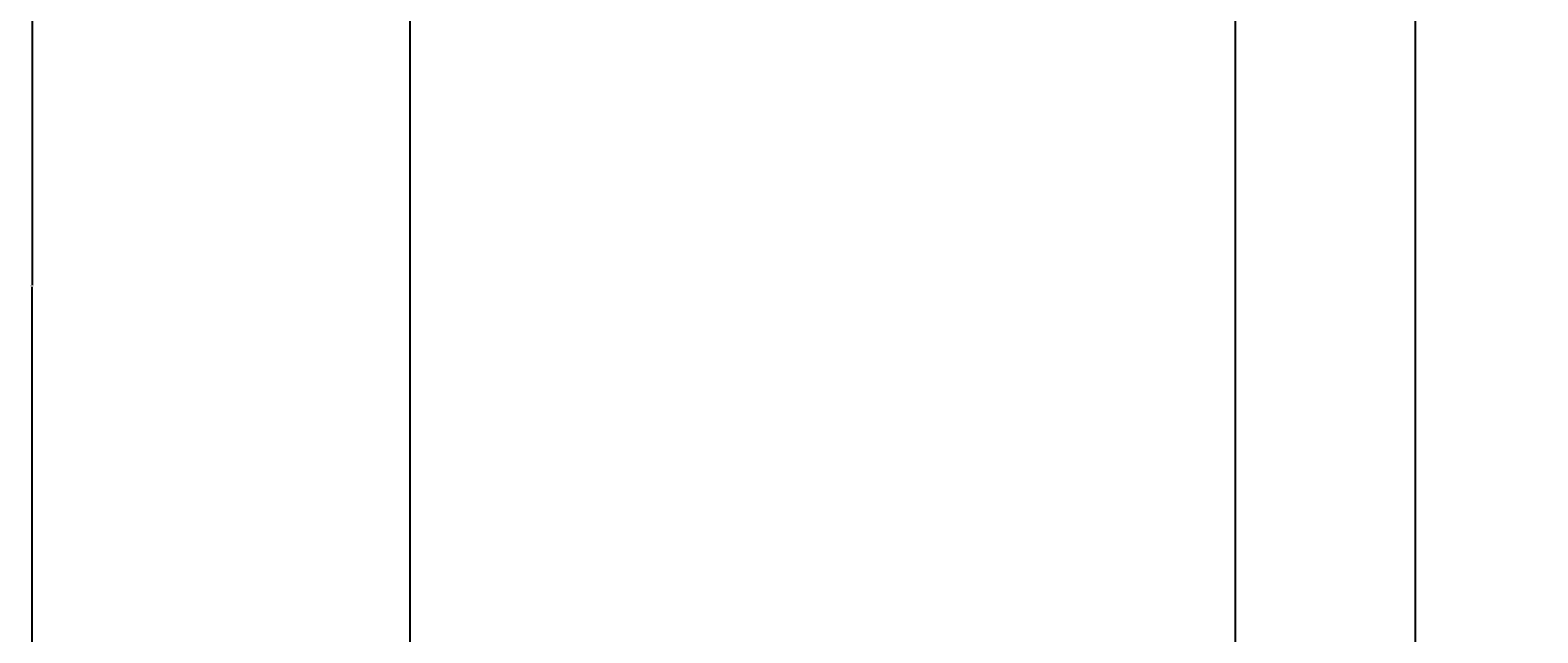
# Model space of a CAD drawing. Units: inches. Extents: x -61 to 1599, y -1316 to 257.
# Tile 42 of 204: x -61 to 240, y -599 to -478. Entities that reach past the tile are written whole.
import ezdxf

# ---------------------------------------------------------------- set-up
doc = ezdxf.new("R2010")
doc.units = ezdxf.units.IN
doc.header["$MEASUREMENT"] = 0
doc.layers.add('A-ANNO-DIMS', color=2, linetype='Continuous', lineweight=18)
doc.styles.get("Standard").update_dxf_attribs({"font": 'arial.ttf'})
doc.dimstyles.get("Standard").update_dxf_attribs({"dimtxt": 0.18, "dimasz": 0.18, "dimexe": 0.18, "dimexo": 0.0625, "dimgap": 0.09, "dimtad": 0, "dimtih": 1, "dimtoh": 1, "dimdec": 0, "dimzin": 0, "dimdsep": 46, "dimlunit": 3, "dimtxsty": 'Standard', "dimcen": 0.09, "dimadec": 0, "dimazin": 0, "dimtfac": 1, "dimtdec": 0, "dimtofl": 0, "dimtmove": 0, "dimatfit": 3, "dimfxl": 1, "dimtolj": 1, "dimtzin": 0, "dimarcsym": 0})

# ---------------------------------------------------------------- blocks, each defined once
blk = doc.blocks.new('*D687')
at = {"layer": 'A-ANNO-DIMS', "color": 0, "lineweight": -2, "transparency": 16777216}
for p, q in [((289.42, 181.68), (-61.08, 181.68)), ((-60.9, 181.5), (-60.9, -528.95)), ((-60.9, -1239.76), (-60.9, -529.32)), ((319.64, -1239.94), (-61.08, -1239.94))]:
    blk.add_line(p, q, dxfattribs=at)
at = {"layer": 'A-ANNO-DIMS', "color": 0, "transparency": 16777216}
for points in [[(-60.93, 181.5), (-60.87, 181.5), (-60.9, 181.68)], [(-60.93, -1239.76), (-60.87, -1239.76), (-60.9, -1239.94)]]:
    blk.add_solid(points, dxfattribs=at)
at = {"layer": 'DEFPOINTS', "color": 0, "transparency": 16777216}
for p in [(289.48, 181.68), (-60.9, -1239.94), (319.7, -1239.94)]:
    blk.add_point(p, dxfattribs=at)
at = {"layer": 'A-ANNO-DIMS', "color": 0, "transparency": 16777216, "insert": (-60.9, -529.13), "char_height": 0.18, "attachment_point": 5}
blk.add_mtext('\\A1;1421.6', dxfattribs=at)
blk = doc.blocks.new('*D692')
at = {"layer": 'A-ANNO-DIMS', "color": 0, "lineweight": -2, "transparency": 16777216}
for p, q in [((14.64, -441.32), (-61.08, -441.32)), ((-60.9, -441.5), (-60.9, -528.95)), ((-60.9, -616.76), (-60.9, -529.32)), ((14.64, -616.94), (-61.08, -616.94))]:
    blk.add_line(p, q, dxfattribs=at)
at = {"layer": 'A-ANNO-DIMS', "color": 0, "transparency": 16777216}
for points in [[(-60.93, -441.5), (-60.87, -441.5), (-60.9, -441.32)], [(-60.93, -616.76), (-60.87, -616.76), (-60.9, -616.94)]]:
    blk.add_solid(points, dxfattribs=at)
at = {"layer": 'DEFPOINTS', "color": 0, "transparency": 16777216}
for p in [(-60.9, -441.32), (14.7, -441.32), (14.7, -616.94)]:
    blk.add_point(p, dxfattribs=at)
at = {"layer": 'A-ANNO-DIMS', "color": 0, "transparency": 16777216, "insert": (-60.9, -529.13), "char_height": 0.18, "attachment_point": 5}
blk.add_mtext('\\A1;175.62', dxfattribs=at)
blk = doc.blocks.new('*D700')
at = {"layer": 'A-ANNO-DIMS', "color": 0, "lineweight": -2, "transparency": 16777216}
for p, q in [((14.7, -616.88), (14.7, 257.46)), ((14.88, 257.28), (96.77, 257.28)), ((179.57, 257.28), (97.68, 257.28)), ((179.75, -616.88), (179.75, 257.46))]:
    blk.add_line(p, q, dxfattribs=at)
at = {"layer": 'A-ANNO-DIMS', "color": 0, "transparency": 16777216}
for points in [[(14.88, 257.31), (14.88, 257.25), (14.7, 257.28)], [(179.57, 257.31), (179.57, 257.25), (179.75, 257.28)]]:
    blk.add_solid(points, dxfattribs=at)
at = {"layer": 'DEFPOINTS', "color": 0, "transparency": 16777216}
for p in [(179.75, 257.28), (14.7, -616.94), (179.75, -616.94)]:
    blk.add_point(p, dxfattribs=at)
at = {"layer": 'A-ANNO-DIMS', "color": 0, "transparency": 16777216, "insert": (97.23, 257.28), "char_height": 0.18, "attachment_point": 5}
blk.add_mtext('\\A1;165.05', dxfattribs=at)
blk = doc.blocks.new('*D701')
at = {"layer": 'A-ANNO-DIMS', "color": 0, "lineweight": -2, "transparency": 16777216}
for p, q in [((215.75, -616.88), (215.75, 257.46)), ((215.93, 257.28), (233.92, 257.28)), ((252.7, 257.28), (234.71, 257.28)), ((252.88, -616.88), (252.88, 257.46))]:
    blk.add_line(p, q, dxfattribs=at)
at = {"layer": 'A-ANNO-DIMS', "color": 0, "transparency": 16777216}
for points in [[(215.93, 257.31), (215.93, 257.25), (215.75, 257.28)], [(252.7, 257.31), (252.7, 257.25), (252.88, 257.28)]]:
    blk.add_solid(points, dxfattribs=at)
at = {"layer": 'DEFPOINTS', "color": 0, "transparency": 16777216}
for p in [(252.88, 257.28), (215.75, -616.94), (252.88, -616.94)]:
    blk.add_point(p, dxfattribs=at)
at = {"layer": 'A-ANNO-DIMS', "color": 0, "transparency": 16777216, "insert": (234.32, 257.28), "char_height": 0.18, "attachment_point": 5}
blk.add_mtext('\\A1;37.13', dxfattribs=at)

msp = doc.modelspace()

# ---------------------------------------------------------------- dimensions: what is measured, and where the dimension line sits
at = {"layer": 'A-ANNO-DIMS'}
for base, p1, p2, picture, middle in [((179.7521, 257.2771), (14.7028, -616.9446), (179.7521, -616.9446), '*D700', (97.2274, 257.2771)), ((252.8825, 257.2771), (215.7521, -616.9446), (252.8825, -616.9446), '*D701', (234.3173, 257.2771))]:
    dim = msp.add_linear_dim(base=base, p1=p1, p2=p2, dimstyle='Standard', override={"dimdec": 2, "dimlfac": 1, "dimrnd": 0, "dimzin": 0, "dimdsep": 46, "dimlunit": 2}, dxfattribs=at)
    dim.commit()
    dim.dimension.update_dxf_attribs({"geometry": picture, "text_midpoint": middle})
for base, p1, p2, override, picture in [((-60.8972, -1239.9446), (289.4807, 181.6771), (319.7028, -1239.9446), {"dimdec": 1, "dimlfac": 1, "dimrnd": 0, "dimzin": 0, "dimdsep": 46, "dimlunit": 2}, '*D687'), ((-60.8972, -441.3229), (14.7028, -616.9446), (14.7028, -441.3229), {"dimdec": 2, "dimlfac": 1, "dimrnd": 0, "dimzin": 0, "dimdsep": 46, "dimlunit": 2}, '*D692')]:
    dim = msp.add_linear_dim(base=base, p1=p1, p2=p2, angle=90, dimstyle='Standard', override=override, dxfattribs=at)
    dim.commit()
    dim.dimension.update_dxf_attribs({"geometry": picture, "text_midpoint": (-60.8972, -529.1337)})

doc.saveas('drawing.dxf')
